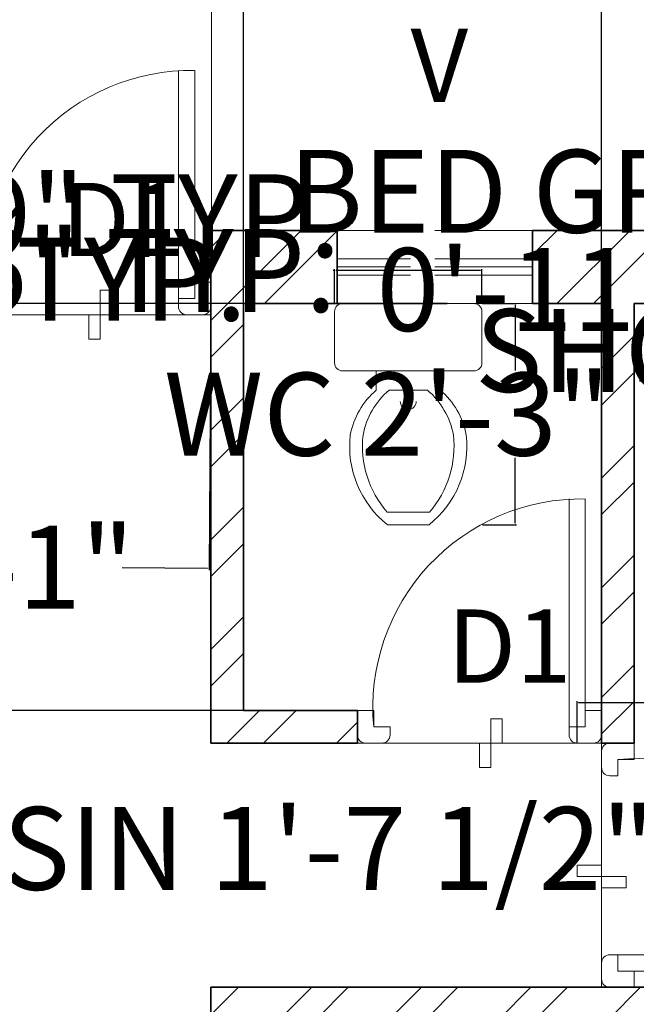
# Model space of a CAD drawing. Units: inches. Extents: x 2379 to 3013, y 1431 to 2110.
# Tile 6 of 10: x 2620 to 2696, y 1927 to 2047. Entities that reach past the tile are written whole.
import ezdxf

# ---------------------------------------------------------------- set-up
doc = ezdxf.new("R2010")
doc.units = ezdxf.units.IN
doc.linetypes.add('ACAD_ISO02W100', pattern=[15, 12, -3])
for name, color, linetype, lineweight in [('A-ANNO-DIMS', 2, 'Continuous', 18), ('A-ANNO-TEXT', 7, 'Continuous', 18), ('A-DOOR', 4, 'Continuous', 18), ('A-FLOR-FIXT', 9, 'Continuous', 18), ('A-FLOR-STRS', 7, 'Continuous', 18), ('A-GLAZ-VENT', 6, 'ACAD_ISO02W100', 13), ('A-WALL-PATT', 8, 'Continuous', 13), ('A_FUR 1', 5, 'Continuous', 5), ('WALL', 7, 'Continuous', 35)]:
    doc.layers.add(name, color=color, linetype=linetype, lineweight=lineweight)
doc.styles.get("Standard").update_dxf_attribs({"font": 'arial.ttf'})
doc.dimstyles.get("Standard").update_dxf_attribs({"dimtxt": 10.18, "dimasz": 0.18, "dimexe": 0.18, "dimexo": 0.0625, "dimgap": 0.09, "dimtad": 0, "dimtih": 1, "dimtoh": 1, "dimdec": 0, "dimzin": 0, "dimdsep": 46, "dimlunit": 3, "dimtxsty": 'Standard', "dimcen": 0.09, "dimadec": 0, "dimazin": 0, "dimtfac": 1, "dimtdec": 0, "dimtofl": 0, "dimtmove": 0, "dimatfit": 3, "dimfxl": 1, "dimtolj": 1, "dimtzin": 0, "dimarcsym": 0})

# ---------------------------------------------------------------- blocks, each defined once
blk = doc.blocks.new('ESTSET')
at = {"layer": 'A_FUR 1'}
for p, q in [((-10.44, 4.1), (-10.44, 32.1)), ((-8.44, 4.1), (-8.44, 32.1)), ((-36.44, 6.1), (-36.44, 3.1)), ((-34.44, 6.1), (-36.44, 6.1)), ((-34.44, 4.1), (-34.44, 6.1)), ((-34.44, 4.1), (-34.44, 6.1)), ((-8.44, 4.1), (-8.44, 6.1)), ((-8.44, 6.1), (-6.44, 6.1)), ((-8.44, 4.1), (-8.44, 6.1)), ((-6.44, 6.1), (-6.44, 3.1)), ((-32.44, 4.1), (-34.44, 4.1)), ((-32.44, 4.1), (-34.44, 4.1)), ((-32.44, 3.1), (-32.44, 4.1)), ((-10.44, 3.1), (-10.44, 4.1)), ((-10.44, 4.1), (-8.44, 4.1)), ((-10.44, 4.1), (-8.44, 4.1)), ((-6.44, 2.1), (-36.44, 2.1)), ((-35.44, 2.1), (-33.44, 2.1)), ((-7.44, 2.1), (-9.44, 2.1))]:
    blk.add_line(p, q, dxfattribs=at)
for points in [[(-21.44, 2.1), (-18.67, 2.1), (-18.67, 5.1), (-20.06, 5.1)], [(-20.06, 5.1), (-20.06, -0.91)], [(-21.44, 2.1), (-21.44, -0.91), (-20.06, -0.91)]]:
    blk.add_lwpolyline(points, dxfattribs=at)
for centre, radius, start, end in [((-8.91, 6.46), 25.64, 88.9606, 185.2816), ((-35.44, 3.1), 1, 180, 270), ((-33.44, 3.1), 1, 270, 0), ((-9.44, 3.1), 1, 180, 270), ((-7.44, 3.1), 1, 270, 0)]:
    blk.add_arc(centre, radius, start, end, dxfattribs=at)
blk = doc.blocks.new('A$C2AC94788')
for p, q in [((0.025, 0.69), (0.435, 0.69)), ((0, 0.505), (0, 0.665)), ((0.46, 0.665), (0.46, 0.505)), ((0.435, 0.48), (0.025, 0.48)), ((0.13, 0.48), (0.13, 0.42)), ((0.33, 0.42), (0.33, 0.48)), ((0.17, 0.42), (0.29, 0.42)), ((0.1641, 0.0392), (0.2959, 0.0392)), ((0.2291, 0.0392), (0.23, 0.0392)), ((0.2309, 0.0392), (0.23, 0.0392)), ((0.165, 0), (0.295, 0))]:
    blk.add_line(p, q)
for centre, radius, start, end in [((0.025, 0.665), 0.025, 90, 180), ((0.435, 0.665), 0.025, 0, 90), ((0.025, 0.505), 0.025, 180, 270), ((0.435, 0.505), 0.025, 270, 0), ((0.2874, 0.2356), 0.2425, 130.4885, 169.445), ((0.3274, 0.2356), 0.2425, 130.4885, 169.445), ((0.1326, 0.2356), 0.2425, 10.555, 49.5115), ((0.1726, 0.2356), 0.2425, 10.555, 49.5115), ((0.23, 0.385), 0.025, 180, 0), ((0.3601, 0.2448), 0.313, 173.5369, 231.4483), ((0.4001, 0.2448), 0.313, 173.5369, 221.0604), ((0.0999, 0.2448), 0.313, 308.5517, 6.4631), ((0.0599, 0.2448), 0.313, 318.9396, 6.4631)]:
    blk.add_arc(centre, radius, start, end)
blk = doc.blocks.new('*D14')
at = {"layer": 'A-ANNO-DIMS', "color": 0, "lineweight": -2, "transparency": 16777216}
for p, q in [((2469.63, 2021.67), (2469.63, 2076.34)), ((2469.81, 2076.16), (2694.9, 2076.16)), ((2937.45, 2076.16), (2712.35, 2076.16)), ((2937.63, 2021.67), (2937.63, 2076.34))]:
    blk.add_line(p, q, dxfattribs=at)
at = {"layer": 'A-ANNO-DIMS', "color": 0, "transparency": 16777216}
for points in [[(2469.81, 2076.19), (2469.81, 2076.13), (2469.63, 2076.16)], [(2937.45, 2076.19), (2937.45, 2076.13), (2937.63, 2076.16)]]:
    blk.add_solid(points, dxfattribs=at)
at = {"layer": 'Defpoints', "color": 0, "transparency": 16777216}
for p in [(2937.63, 2076.16), (2469.63, 2021.61), (2937.63, 2021.61)]:
    blk.add_point(p, dxfattribs=at)
at = {"layer": 'A-ANNO-DIMS', "color": 0, "transparency": 16777216, "insert": (2703.63, 2076.16), "char_height": 10.18, "attachment_point": 5}
blk.add_mtext("\\A1;39'", dxfattribs=at)
blk = doc.blocks.new('VENT-24IN')
for p, q in [((24, 5.5), (0, 5.5)), ((24, 4.5), (0, 4.5)), ((24, 3.5), (0, 3.5))]:
    blk.add_line(p, q)
blk.add_lwpolyline([(0, 9), (0, 0), (24, 0), (24, 9)], close=True)
blk = doc.blocks.new('*D20')
at = {"layer": 'A-ANNO-DIMS', "color": 0, "lineweight": -2, "transparency": 16777216}
for p, q in [((2588.15, 2021.61), (2586.23, 2021.61)), ((2586.41, 2021.43), (2586.41, 2020.97)), ((2588.15, 2009.61), (2586.23, 2009.61)), ((2586.41, 2009.79), (2586.41, 2010.25))]:
    blk.add_line(p, q, dxfattribs=at)
at = {"layer": 'A-ANNO-DIMS', "color": 0, "transparency": 16777216}
for points in [[(2586.38, 2021.43), (2586.44, 2021.43), (2586.41, 2021.61)], [(2586.38, 2009.79), (2586.44, 2009.79), (2586.41, 2009.61)]]:
    blk.add_solid(points, dxfattribs=at)
at = {"layer": 'Defpoints', "color": 0, "transparency": 16777216}
for p in [(2586.41, 2021.61), (2588.21, 2021.61), (2588.21, 2009.61)]:
    blk.add_point(p, dxfattribs=at)
at = {"layer": 'A-ANNO-DIMS', "color": 0, "transparency": 16777216, "insert": (2586.41, 2015.61), "char_height": 10.18, "attachment_point": 5}
blk.add_mtext('\\A1;COLUMN 1\'-0" TYP.', dxfattribs=at)
blk = doc.blocks.new('*D21')
at = {"layer": 'A-ANNO-DIMS', "color": 0, "lineweight": -2, "transparency": 16777216}
for p, q in [((2588.21, 2021.67), (2588.21, 2023.59)), ((2588.39, 2023.41), (2597.03, 2023.41)), ((2597.21, 2021.67), (2597.21, 2023.59)), ((2597.21, 2023.41), (2597.39, 2023.41))]:
    blk.add_line(p, q, dxfattribs=at)
at = {"layer": 'A-ANNO-DIMS', "color": 0, "transparency": 16777216}
for points in [[(2588.39, 2023.44), (2588.39, 2023.38), (2588.21, 2023.41)], [(2597.03, 2023.44), (2597.03, 2023.38), (2597.21, 2023.41)]]:
    blk.add_solid(points, dxfattribs=at)
at = {"layer": 'Defpoints', "color": 0, "transparency": 16777216}
for p in [(2597.21, 2023.41), (2588.21, 2021.61), (2597.21, 2021.61)]:
    blk.add_point(p, dxfattribs=at)
at = {"layer": 'A-ANNO-DIMS', "color": 0, "transparency": 16777216, "insert": (2628.51, 2023.41), "char_height": 10.18, "attachment_point": 5}
blk.add_mtext('\\A1;0\'-9" TYP.', dxfattribs=at)
blk = doc.blocks.new('*D26')
at = {"layer": 'A-ANNO-DIMS', "color": 0, "lineweight": -2, "transparency": 16777216}
for p, q in [((2688.62, 1958.67), (2688.62, 1963.76)), ((2688.8, 1963.58), (2721.58, 1963.58)), ((2721.76, 1958.67), (2721.76, 1963.76)), ((2721.76, 1963.58), (2721.94, 1963.58))]:
    blk.add_line(p, q, dxfattribs=at)
at = {"layer": 'A-ANNO-DIMS', "color": 0, "transparency": 16777216}
for points in [[(2688.8, 1963.61), (2688.8, 1963.55), (2688.62, 1963.58)], [(2721.58, 1963.61), (2721.58, 1963.55), (2721.76, 1963.58)]]:
    blk.add_solid(points, dxfattribs=at)
at = {"layer": 'Defpoints', "color": 0, "transparency": 16777216}
for p in [(2721.76, 1963.58), (2688.62, 1958.61), (2721.76, 1958.61)]:
    blk.add_point(p, dxfattribs=at)
at = {"layer": 'A-ANNO-DIMS', "color": 0, "transparency": 16777216, "insert": (2787.18, 1963.58), "char_height": 10.18, "attachment_point": 5}
blk.add_mtext('\\A1;DOOR D1 2\'-9" TYP.', dxfattribs=at)
blk = doc.blocks.new('*D30')
at = {"layer": 'A-ANNO-DIMS', "color": 0, "lineweight": -2, "transparency": 16777216}
for p, q in [((2800.26, 2026.41), (2800.08, 2026.41)), ((2800.26, 2011.63), (2800.26, 2026.59)), ((2899.08, 2026.41), (2800.44, 2026.41)), ((2899.26, 2011.63), (2899.26, 2026.59))]:
    blk.add_line(p, q, dxfattribs=at)
at = {"layer": 'A-ANNO-DIMS', "color": 0, "transparency": 16777216}
for points in [[(2800.44, 2026.44), (2800.44, 2026.38), (2800.26, 2026.41)], [(2899.08, 2026.44), (2899.08, 2026.38), (2899.26, 2026.41)]]:
    blk.add_solid(points, dxfattribs=at)
at = {"layer": 'Defpoints', "color": 0, "transparency": 16777216}
for p in [(2800.26, 2026.41), (2800.26, 2011.56), (2899.26, 2011.56)]:
    blk.add_point(p, dxfattribs=at)
at = {"layer": 'A-ANNO-DIMS', "color": 0, "transparency": 16777216, "insert": (2724.54, 2026.41), "char_height": 10.18, "attachment_point": 5}
blk.add_mtext('\\A1;BED GROUP 8\'-3" TYP.', dxfattribs=at)
blk = doc.blocks.new('*D40')
at = {"layer": 'A-ANNO-DIMS', "color": 0, "lineweight": -2, "transparency": 16777216}
for p, q in [((2677, 2012.61), (2681.19, 2012.61)), ((2681.01, 2012.43), (2681.01, 2004.38)), ((2681.01, 1985.62), (2681.01, 1993.67)), ((2677, 1985.44), (2681.19, 1985.44))]:
    blk.add_line(p, q, dxfattribs=at)
at = {"layer": 'A-ANNO-DIMS', "color": 0, "transparency": 16777216}
for points in [[(2680.98, 2012.43), (2681.04, 2012.43), (2681.01, 2012.61)], [(2680.98, 1985.62), (2681.04, 1985.62), (2681.01, 1985.44)]]:
    blk.add_solid(points, dxfattribs=at)
at = {"layer": 'Defpoints', "color": 0, "transparency": 16777216}
for p in [(2676.93, 2012.61), (2681.01, 2012.61), (2676.93, 1985.44)]:
    blk.add_point(p, dxfattribs=at)
at = {"layer": 'A-ANNO-DIMS', "color": 0, "transparency": 16777216, "insert": (2681.01, 1999.02), "char_height": 10.18, "attachment_point": 5}
blk.add_mtext('\\A1;WC 2\'-3" TYP.', dxfattribs=at)
blk = doc.blocks.new('*D41')
at = {"layer": 'A-ANNO-DIMS', "color": 0, "lineweight": -2, "transparency": 16777216}
for p, q in [((2658.82, 2016.68), (2658.64, 2016.68)), ((2658.82, 2012.67), (2658.82, 2016.86)), ((2676.75, 2016.68), (2659, 2016.68)), ((2676.93, 2012.67), (2676.93, 2016.86))]:
    blk.add_line(p, q, dxfattribs=at)
at = {"layer": 'A-ANNO-DIMS', "color": 0, "transparency": 16777216}
for points in [[(2659, 2016.71), (2659, 2016.65), (2658.82, 2016.68)], [(2676.75, 2016.71), (2676.75, 2016.65), (2676.93, 2016.68)]]:
    blk.add_solid(points, dxfattribs=at)
at = {"layer": 'Defpoints', "color": 0, "transparency": 16777216}
for p in [(2658.82, 2016.68), (2658.82, 2012.61), (2676.93, 2012.61)]:
    blk.add_point(p, dxfattribs=at)
at = {"layer": 'A-ANNO-DIMS', "color": 0, "transparency": 16777216, "insert": (2628, 2016.68), "char_height": 10.18, "attachment_point": 5}
blk.add_mtext('\\A1;1\'-6" TYP.', dxfattribs=at)
blk = doc.blocks.new('*D42')
at = {"layer": 'A-ANNO-DIMS', "color": 0, "lineweight": -2, "transparency": 16777216}
for p, q in [((2731.29, 1945.67), (2731.11, 1945.67)), ((2731.29, 1942.77), (2731.29, 1945.85)), ((2750.86, 1945.67), (2731.47, 1945.67)), ((2751.04, 1942.77), (2751.04, 1945.85))]:
    blk.add_line(p, q, dxfattribs=at)
at = {"layer": 'A-ANNO-DIMS', "color": 0, "transparency": 16777216}
for points in [[(2731.47, 1945.7), (2731.47, 1945.64), (2731.29, 1945.67)], [(2750.86, 1945.7), (2750.86, 1945.64), (2751.04, 1945.67)]]:
    blk.add_solid(points, dxfattribs=at)
at = {"layer": 'Defpoints', "color": 0, "transparency": 16777216}
for p in [(2731.29, 1945.67), (2731.29, 1942.71), (2751.04, 1942.71)]:
    blk.add_point(p, dxfattribs=at)
at = {"layer": 'A-ANNO-DIMS', "color": 0, "transparency": 16777216, "insert": (2665.05, 1945.67), "char_height": 10.18, "attachment_point": 5}
blk.add_mtext('\\A1;BASIN 1\'-7 1/2" TYP.', dxfattribs=at)
blk = doc.blocks.new('*D46')
at = {"layer": 'A-ANNO-DIMS', "color": 0, "lineweight": -2, "transparency": 16777216}
for p, q in [((2736.09, 2012.61), (2737.93, 2012.61)), ((2737.75, 2012.43), (2737.75, 2012.2)), ((2736.09, 2001.09), (2737.93, 2001.09)), ((2737.75, 2001.27), (2737.75, 2001.49))]:
    blk.add_line(p, q, dxfattribs=at)
at = {"layer": 'A-ANNO-DIMS', "color": 0, "transparency": 16777216}
for points in [[(2737.72, 2012.43), (2737.78, 2012.43), (2737.75, 2012.61)], [(2737.72, 2001.27), (2737.78, 2001.27), (2737.75, 2001.09)]]:
    blk.add_solid(points, dxfattribs=at)
at = {"layer": 'Defpoints', "color": 0, "transparency": 16777216}
for p in [(2736.02, 2012.61), (2737.75, 2012.61), (2736.02, 2001.09)]:
    blk.add_point(p, dxfattribs=at)
at = {"layer": 'A-ANNO-DIMS', "color": 0, "transparency": 16777216, "insert": (2737.75, 2006.85), "char_height": 10.18, "attachment_point": 5}
blk.add_mtext('\\A1;SHOWER 0\'-11 1/2"', dxfattribs=at)
blk = doc.blocks.new('*D47')
at = {"layer": 'A-ANNO-DIMS', "color": 0, "lineweight": -2, "transparency": 16777216}
for p, q in [((2724.76, 2014.34), (2724.58, 2014.34)), ((2724.76, 2012.67), (2724.76, 2014.52)), ((2735.84, 2014.34), (2724.94, 2014.34)), ((2736.02, 2012.67), (2736.02, 2014.52))]:
    blk.add_line(p, q, dxfattribs=at)
at = {"layer": 'A-ANNO-DIMS', "color": 0, "transparency": 16777216}
for points in [[(2724.94, 2014.37), (2724.94, 2014.31), (2724.76, 2014.34)], [(2735.84, 2014.37), (2735.84, 2014.31), (2736.02, 2014.34)]]:
    blk.add_solid(points, dxfattribs=at)
at = {"layer": 'Defpoints', "color": 0, "transparency": 16777216}
for p in [(2724.76, 2014.34), (2724.76, 2012.61), (2736.02, 2012.61)]:
    blk.add_point(p, dxfattribs=at)
at = {"layer": 'A-ANNO-DIMS', "color": 0, "transparency": 16777216, "insert": (2695.15, 2014.34), "char_height": 10.18, "attachment_point": 5}
blk.add_mtext('\\A1;0\'-11 1/2"', dxfattribs=at)
blk = doc.blocks.new('*D55')
at = {"layer": 'A-ANNO-DIMS', "color": 0, "lineweight": -2, "transparency": 16777216}
for p, q in [((2647.63, 2012.67), (2647.63, 2094.64)), ((2647.81, 2094.46), (2656.01, 2094.46)), ((2691.45, 2094.46), (2683.25, 2094.46)), ((2691.63, 2012.67), (2691.63, 2094.64))]:
    blk.add_line(p, q, dxfattribs=at)
at = {"layer": 'A-ANNO-DIMS', "color": 0, "transparency": 16777216}
for points in [[(2647.81, 2094.49), (2647.81, 2094.43), (2647.63, 2094.46)], [(2691.45, 2094.49), (2691.45, 2094.43), (2691.63, 2094.46)]]:
    blk.add_solid(points, dxfattribs=at)
at = {"layer": 'Defpoints', "color": 0, "transparency": 16777216}
for p in [(2691.63, 2094.46), (2647.63, 2012.61), (2691.63, 2012.61)]:
    blk.add_point(p, dxfattribs=at)
at = {"layer": 'A-ANNO-DIMS', "color": 0, "transparency": 16777216, "insert": (2669.63, 2094.46), "char_height": 10.18, "attachment_point": 5}
blk.add_mtext('\\A1;3\'-8"', dxfattribs=at)
blk = doc.blocks.new('*D56')
at = {"layer": 'A-ANNO-DIMS', "color": 0, "lineweight": -2, "transparency": 16777216}
for p, q in [((2647.57, 2012.61), (2422.39, 2012.61)), ((2422.57, 2012.43), (2422.57, 1992.81)), ((2422.57, 1962.79), (2422.57, 1982.41)), ((2647.57, 1962.61), (2422.39, 1962.61))]:
    blk.add_line(p, q, dxfattribs=at)
at = {"layer": 'A-ANNO-DIMS', "color": 0, "transparency": 16777216}
for points in [[(2422.54, 2012.43), (2422.6, 2012.43), (2422.57, 2012.61)], [(2422.54, 1962.79), (2422.6, 1962.79), (2422.57, 1962.61)]]:
    blk.add_solid(points, dxfattribs=at)
at = {"layer": 'Defpoints', "color": 0, "transparency": 16777216}
for p in [(2647.63, 2012.61), (2422.57, 1962.61), (2647.63, 1962.61)]:
    blk.add_point(p, dxfattribs=at)
at = {"layer": 'A-ANNO-DIMS', "color": 0, "transparency": 16777216, "insert": (2422.57, 1987.61), "char_height": 10.18, "attachment_point": 5}
blk.add_mtext('\\A1;4\'-2"', dxfattribs=at)
blk = doc.blocks.new('*D70')
at = {"layer": 'A-ANNO-DIMS', "color": 0, "lineweight": -2, "transparency": 16777216}
for p, q in [((2594.63, 2012.55), (2594.39, 1980.23)), ((2643.63, 2012.19), (2643.39, 1979.87)), ((2594.57, 1980.41), (2605.07, 1980.33)), ((2643.21, 1980.05), (2632.72, 1980.13))]:
    blk.add_line(p, q, dxfattribs=at)
at = {"layer": 'A-ANNO-DIMS', "color": 0, "transparency": 16777216}
for points in [[(2594.57, 1980.44), (2594.57, 1980.38), (2594.39, 1980.41)], [(2643.21, 1980.08), (2643.21, 1980.02), (2643.39, 1980.05)]]:
    blk.add_solid(points, dxfattribs=at)
at = {"layer": 'Defpoints', "color": 0, "transparency": 16777216}
for p in [(2594.63, 2012.61), (2643.63, 2012.25), (2594.39, 1980.41)]:
    blk.add_point(p, dxfattribs=at)
at = {"layer": 'A-ANNO-DIMS', "color": 0, "transparency": 16777216, "insert": (2618.89, 1980.23), "char_height": 10.18, "attachment_point": 5}
blk.add_mtext('\\A1;4\'-1"', dxfattribs=at)

msp = doc.modelspace()

# ---------------------------------------------------------------- hatches: boundary and pattern name
at = {"layer": 'A-WALL-PATT'}
h = msp.add_hatch(dxfattribs=at)
h.set_pattern_fill('ANSI32', color=256)
h.paths.add_polyline_path([(2925.63, 1862.61), (2815.63, 1862.61), (2815.63, 1858.61), (2827.63, 1858.61), (2827.63, 1810.61), (2815.63, 1810.61), (2815.63, 1806.61), (2850.78, 1806.61), (2850.78, 1810.61), (2831.63, 1810.61), (2831.63, 1858.61), (2925.63, 1858.61)])
h.paths.add_polyline_path([(2925.63, 1810.61), (2880.78, 1810.61), (2880.78, 1806.61), (2925.63, 1806.61)], flags=17)
h.paths.add_polyline_path([(2633.75, 1660.61), (2594.63, 1660.61), (2481.63, 1660.61), (2481.63, 1651.61), (2588.63, 1651.61), (2588.63, 1570.61), (2624.28, 1570.61), (2624.28, 1574.61), (2592.63, 1574.61), (2592.63, 1651.61), (2633.75, 1651.61)])
h.paths.add_polyline_path([(2594.63, 1809.61), (2481.63, 1809.61), (2481.63, 1805.61), (2594.63, 1805.61)])
h.paths.add_polyline_path([(2594.63, 2012.61), (2597.21, 2012.61), (2597.21, 2021.61), (2588.21, 2021.61), (2588.21, 2012.61), (2590.63, 2012.61), (2590.63, 1845.61), (2594.63, 1845.61)])
h.paths.add_polyline_path([(2767.63, 2012.61), (2770.27, 2012.61), (2770.27, 2021.61), (2761.27, 2021.61), (2761.27, 2012.61), (2763.63, 2012.61), (2763.63, 1928.61), (2691.63, 1928.61), (2643.63, 1928.61), (2643.63, 1924.61), (2691.63, 1924.61), (2763.63, 1924.61), (2763.63, 1858.61), (2779.63, 1858.61), (2779.63, 1862.61), (2767.63, 1862.61)])
h.paths.add_polyline_path([(2613.63, 2012.61), (2613.63, 2021.61), (2597.21, 2021.61), (2597.21, 2012.61)])
h.paths.add_polyline_path([(2508.33, 2012.61), (2508.33, 2021.61), (2478.63, 2021.61), (2478.63, 2012.61)])
h.paths.add_polyline_path([(2556.33, 2021.61), (2556.33, 2012.61), (2588.21, 2012.61), (2588.21, 2021.61)])
h.paths.add_polyline_path([(2659.15, 2012.61), (2659.15, 2021.61), (2643.63, 2021.61), (2643.63, 1958.61), (2661.63, 1958.61), (2661.63, 1962.61), (2647.63, 1962.61), (2647.63, 2012.61)])
h.paths.add_polyline_path([(2714.17, 2012.61), (2714.17, 2021.61), (2683.15, 2021.61), (2683.15, 2012.61), (2691.63, 2012.61), (2691.63, 1958.61), (2695.63, 1958.61), (2695.63, 2012.61)])
h.paths.add_polyline_path([(2738.17, 2021.61), (2738.17, 2012.61), (2761.27, 2012.61), (2761.27, 2021.61)])
h.paths.add_polyline_path([(2820.76, 2012.61), (2820.76, 2021.61), (2770.27, 2021.61), (2770.27, 2012.61)])
h.paths.add_polyline_path([(2868.76, 2021.61), (2868.76, 2012.61), (2928.63, 2012.61), (2928.63, 2021.61)])
h.paths.add_polyline_path([(2928.63, 1962.9), (2937.63, 1962.9), (2937.63, 2009.61), (2928.63, 2009.61)])
h.paths.add_polyline_path([(2937.63, 1914.9), (2928.63, 1914.9), (2928.63, 1863.8), (2937.63, 1863.8)])
h.paths.add_polyline_path([(2928.63, 1846.59), (2937.63, 1846.59), (2937.63, 1854.8), (2928.63, 1854.8)])
h.paths.add_polyline_path([(2937.63, 1822.59), (2928.63, 1822.59), (2928.63, 1813.62), (2937.63, 1813.62)])
h.paths.add_polyline_path([(2928.63, 1778.48), (2937.63, 1778.48), (2937.63, 1813.62), (2928.63, 1813.62), (2928.63, 1810.61), (2925.63, 1810.61), (2925.63, 1806.61), (2928.63, 1806.61)])
h.paths.add_polyline_path([(2816.22, 1651.61), (2816.22, 1660.61), (2767.63, 1660.61), (2767.63, 1806.61), (2779.63, 1806.61), (2779.63, 1810.61), (2763.63, 1810.61), (2763.63, 1660.61), (2688.63, 1660.61), (2688.63, 1810.61), (2684.63, 1810.61), (2684.63, 1660.61), (2669.75, 1660.61), (2669.75, 1651.61), (2763.63, 1651.61), (2763.63, 1574.61), (2672.28, 1574.61), (2672.28, 1570.61), (2767.63, 1570.61), (2767.63, 1651.61)])
h.paths.add_polyline_path([(2864.22, 1660.61), (2864.22, 1651.61), (2937.63, 1651.61), (2937.63, 1730.48), (2928.63, 1730.48), (2928.63, 1660.61)])
h.paths.add_polyline_path([(2469.63, 1975.19), (2478.63, 1975.19), (2478.63, 2009.61), (2469.63, 2009.61)])
h.paths.add_polyline_path([(2478.63, 1927.19), (2469.63, 1927.19), (2469.63, 1811.02), (2478.63, 1811.02)])
h.paths.add_polyline_path([(2469.63, 1758.04), (2478.63, 1758.04), (2478.63, 1802.02), (2469.63, 1802.02)])
h.paths.add_polyline_path([(2478.63, 1710.04), (2469.63, 1710.04), (2469.63, 1660.61), (2478.63, 1660.61)])

# ---------------------------------------------------------------- linework, layer by layer
at = {"layer": 'A-FLOR-STRS'}
msp.add_line((2643.7, 2021.61), (2643.7, 2062.26), dxfattribs=at)
at = {"layer": 'WALL'}
for p, q in [((2643.63, 2021.61), (2643.63, 1958.61)), ((2643.63, 2021.61), (2659.15, 2021.61)), ((2659.15, 2012.61), (2659.15, 2021.61)), ((2683.15, 2012.61), (2683.15, 2021.61)), ((2683.15, 2021.61), (2714.17, 2021.61)), ((2647.63, 2012.61), (2647.63, 1962.61)), ((2647.63, 2012.61), (2672.66, 2012.61)), ((2683.15, 2012.61), (2691.63, 2012.61)), ((2691.63, 2012.61), (2691.63, 1958.61)), ((2695.63, 2012.61), (2695.63, 1958.61)), ((2695.63, 2012.61), (2717.56, 2012.61)), ((2661.63, 1962.61), (2647.63, 1962.61)), ((2661.63, 1962.61), (2661.63, 1958.61)), ((2661.63, 1958.61), (2643.63, 1958.61)), ((2691.63, 1958.61), (2695.63, 1958.61)), ((2643.63, 1928.61), (2691.63, 1928.61)), ((2643.63, 1928.61), (2643.63, 1924.61)), ((2691.63, 1928.61), (2763.63, 1928.61))]:
    msp.add_line(p, q, dxfattribs=at)

# ---------------------------------------------------------------- block references
at = {"layer": 'A-DOOR'}
for p in [(2650.07, 2009.15), (2698.07, 1956.51)]:
    msp.add_blockref('ESTSET', p, dxfattribs=at)
at = {"layer": 'A-DOOR', "rotation": 270}
msp.add_blockref('ESTSET', (2689.53, 1922.16), dxfattribs=at)
at = {"layer": 'A-FLOR-FIXT', "xscale": -39.375, "yscale": 39.375, "zscale": 39.375}
msp.add_blockref('A$C2AC94788', (2676.93, 1985.44), dxfattribs=at)
at = {"layer": 'A-GLAZ-VENT'}
msp.add_blockref('VENT-24IN', (2659.15, 2012.61), dxfattribs=at)

# ---------------------------------------------------------------- texts
at = {"layer": 'A-ANNO-TEXT', "char_height": 9, "attachment_point": 1}
for s, insert in [('V', (2668.16, 2046.38)), ('D1', (2625.23, 2027.44)), ('D1', (2672.68, 1975.03))]:
    msp.add_mtext_dynamic_manual_height_columns(s, width=106.8919, gutter_width=12.5, heights=[0], dxfattribs=dict(at, insert=insert))

# ---------------------------------------------------------------- dimensions: what is measured, and where the dimension line sits
at = {"layer": 'A-ANNO-DIMS'}
for base, p1, p2, override, picture, middle in [((2691.63, 2094.46), (2647.63, 2012.61), (2691.63, 2012.61), {"dimdec": 1, "dimlfac": 1, "dimrnd": 0, "dimzin": 1, "dimdsep": 46, "dimlunit": 4, "dimfrac": 2}, '*D55', (2669.63, 2094.46)), ((2937.63, 2076.16), (2469.63, 2021.61), (2937.63, 2021.61), {"dimclrd": 0, "dimclre": 0, "dimclrt": 0}, '*D14', (2703.63, 2076.16))]:
    dim = msp.add_linear_dim(base=base, p1=p1, p2=p2, dimstyle='Standard', override=override, dxfattribs=at)
    dim.commit()
    dim.dimension.update_dxf_attribs({"geometry": picture, "text_midpoint": middle})
for base, p1, p2, angle, text, picture, middle in [((2800.26, 2026.41), (2899.26, 2011.56), (2800.26, 2011.56), 180, 'BED GROUP <> TYP.', '*D30', (2724.54, 2026.41)), ((2586.41, 2021.61), (2588.21, 2009.61), (2588.21, 2021.61), 90, 'COLUMN <> TYP.', '*D20', (2586.41, 2015.61)), ((2658.82, 2016.68), (2676.93, 2012.61), (2658.82, 2012.61), 180, '<> TYP.', '*D41', (2628, 2016.68)), ((2737.75, 2012.61), (2736.02, 2001.09), (2736.02, 2012.61), 90, 'SHOWER <>', '*D46', (2737.75, 2006.85)), ((2681.01, 2012.61), (2676.93, 1985.44), (2676.93, 2012.61), 90, 'WC <> TYP.', '*D40', (2681.01, 1999.02)), ((2731.2925, 1945.6679), (2751.0381, 1942.706), (2731.2925, 1942.706), 180, 'BASIN <> TYP.', '*D42', (2665.0469, 1945.6679))]:
    dim = msp.add_linear_dim(base=base, p1=p1, p2=p2, angle=angle, text=text, dimstyle='Standard', override={"dimdec": 1, "dimlfac": 1, "dimrnd": 0, "dimzin": 1, "dimdsep": 46, "dimlunit": 4, "dimfrac": 2}, dxfattribs=at)
    dim.commit()
    dim.dimension.update_dxf_attribs({"geometry": picture, "text_midpoint": middle})
for base, p1, p2, text, picture, middle in [((2597.21, 2023.41), (2588.21, 2021.61), (2597.21, 2021.61), '<> TYP.', '*D21', (2628.51, 2023.41)), ((2721.76, 1963.58), (2688.62, 1958.61), (2721.76, 1958.61), 'DOOR D1 <> TYP.', '*D26', (2787.18, 1963.58))]:
    dim = msp.add_linear_dim(base=base, p1=p1, p2=p2, text=text, dimstyle='Standard', override={"dimdec": 1, "dimlfac": 1, "dimrnd": 0, "dimzin": 1, "dimdsep": 46, "dimlunit": 4, "dimfrac": 2}, dxfattribs=at)
    dim.commit()
    dim.dimension.update_dxf_attribs({"geometry": picture, "text_midpoint": middle})
for base, p1, p2, angle, picture, middle in [((2724.76, 2014.34), (2736.02, 2012.61), (2724.76, 2012.61), 180, '*D47', (2695.15, 2014.34)), ((2422.57, 1962.61), (2647.63, 2012.61), (2647.63, 1962.61), 90, '*D56', (2422.57, 1987.61)), ((2594.39, 1980.41), (2643.63, 2012.25), (2594.63, 2012.61), 179.5794, '*D70', (2618.89, 1980.23))]:
    dim = msp.add_linear_dim(base=base, p1=p1, p2=p2, angle=angle, dimstyle='Standard', override={"dimdec": 1, "dimlfac": 1, "dimrnd": 0, "dimzin": 1, "dimdsep": 46, "dimlunit": 4, "dimfrac": 2}, dxfattribs=at)
    dim.commit()
    dim.dimension.update_dxf_attribs({"geometry": picture, "text_midpoint": middle})

doc.saveas('drawing.dxf')
